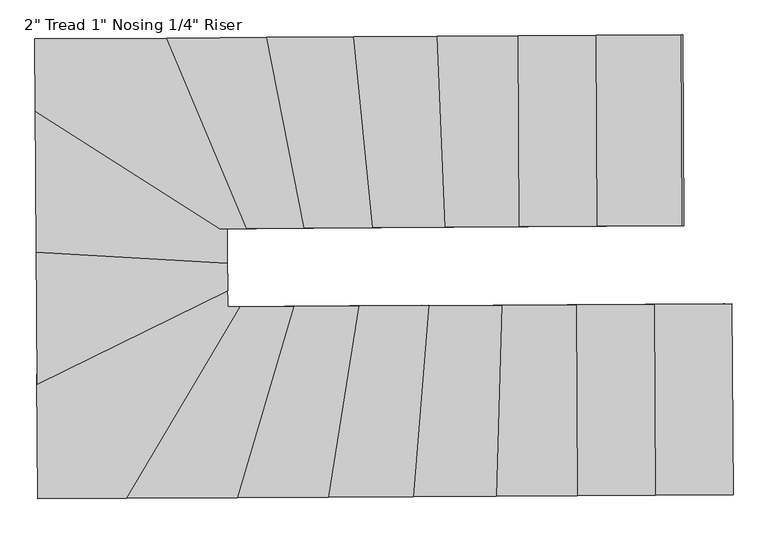
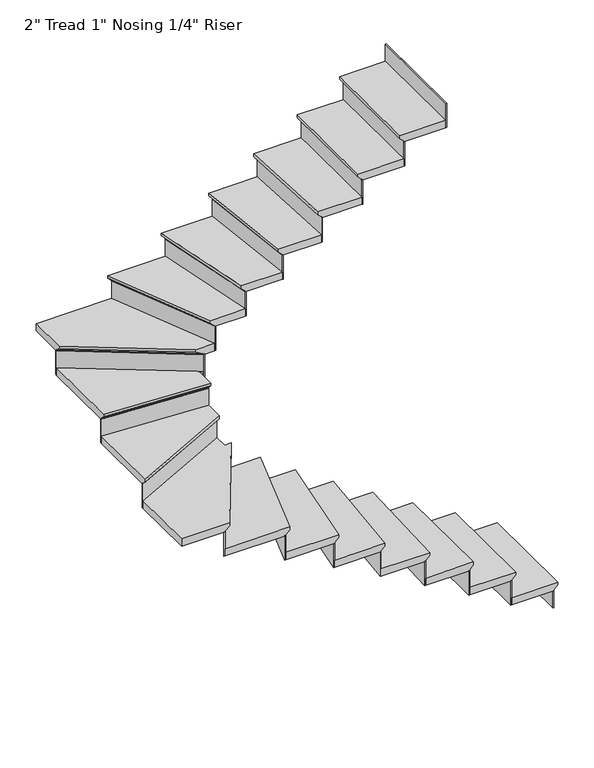
"""IFC4 building model written with IfcOpenShell, lengths in millimetres: stair flight geometry."""

from ifc_helpers import new_model, si_unit, origin, place, context, project, spatial, faceted_brep, source, transform, mapped, element, save


def stair_flight_f68b1b91(model_context):
    return source(origin(), model_context, "Body", "Brep", [
        faceted_brep([(-120.6930289, -3539.621908, 9751.4833333), (-120.6930289, -3539.621908, 9770.5333333), (-116.4891496, -4225.4090232, 9770.5333333), (-116.4891496, -4225.4090232, 9751.4833333), (-146.0925517, -3539.7776072, 9726.0833333), (-141.8886723, -4225.5647224, 9726.0833333), (-425.4873024, -3541.4902988, 9770.5333333), (-421.283423, -4227.277414, 9770.5333333), (-141.8886723, -4225.5647224, 9719.7333333), (-421.283423, -4227.277414, 9719.7333333), (-425.4873024, -3541.4902988, 9719.7333333), (-146.0925517, -3539.7776072, 9719.7333333)], [[[0, 1, 2, 3]], [[4, 0, 3, 5]], [[2, 1, 6, 7]], [[8, 9, 10, 11]], [[2, 7, 9, 8, 5, 3]], [[8, 11, 4, 5]], [[6, 1, 0, 4, 11, 10]], [[7, 6, 10, 9]]]),
        faceted_brep([(-146.0925517, -3539.7776072, 9719.7333333), (-146.0925517, -3539.7776072, 9601.2), (-152.4424324, -3539.816532, 9601.2), (-152.4424324, -3539.816532, 9719.7333333), (-141.8886723, -4225.5647224, 9719.7333333), (-148.238553, -4225.6036472, 9719.7333333), (-148.238553, -4225.6036472, 9601.2), (-141.8886723, -4225.5647224, 9601.2)], [[[0, 1, 2, 3]], [[4, 5, 6, 7]], [[1, 0, 4, 7]], [[2, 1, 7, 6]], [[3, 2, 6, 5]], [[0, 3, 5, 4]]]),
        faceted_brep([(-425.4873024, -3541.4902988, 9889.0666667), (-425.4873024, -3541.4902988, 9719.7333333), (-431.8371831, -3541.5292236, 9719.7333333), (-431.8371831, -3541.5292236, 9889.0666667), (-421.283423, -4227.277414, 9889.0666667), (-427.6333037, -4227.3163388, 9889.0666667), (-427.6333037, -4227.3163388, 9719.7333333), (-421.283423, -4227.277414, 9719.7333333)], [[[0, 1, 2, 3]], [[4, 5, 6, 7]], [[1, 0, 4, 7]], [[2, 1, 7, 6]], [[3, 2, 6, 5]], [[0, 3, 5, 4]]]),
        faceted_brep([(-395.8839002, -4227.1217148, 9939.8666667), (-400.0877796, -3541.3345996, 9939.8666667), (-704.882053, -3543.2029904, 9939.8666667), (-700.6781736, -4228.9901056, 9939.8666667), (-421.283423, -4227.277414, 9889.0666667), (-700.6781736, -4228.9901056, 9889.0666667), (-704.882053, -3543.2029904, 9889.0666667), (-425.4873024, -3541.4902988, 9889.0666667), (-421.283423, -4227.277414, 9895.4166667), (-395.8839002, -4227.1217148, 9920.8166667), (-425.4873024, -3541.4902988, 9895.4166667), (-400.0877796, -3541.3345996, 9920.8166667)], [[[0, 1, 2, 3]], [[4, 5, 6, 7]], [[0, 3, 5, 4, 8, 9]], [[4, 7, 10, 8]], [[2, 1, 11, 10, 7, 6]], [[3, 2, 6, 5]], [[11, 1, 0, 9]], [[10, 11, 9, 8]]]),
        faceted_brep([(-704.882053, -3543.2029904, 10058.4), (-704.882053, -3543.2029904, 9889.0666667), (-711.2319337, -3543.2419152, 9889.0666667), (-711.2319337, -3543.2419152, 10058.4), (-700.6781736, -4228.9901056, 10058.4), (-707.0280543, -4229.0290304, 10058.4), (-707.0280543, -4229.0290304, 9889.0666667), (-700.6781736, -4228.9901056, 9889.0666667)], [[[0, 1, 2, 3]], [[4, 5, 6, 7]], [[1, 0, 4, 7]], [[2, 1, 7, 6]], [[3, 2, 6, 5]], [[0, 3, 5, 4]]]),
        faceted_brep([(-675.2786508, -4228.8344064, 10109.2), (-679.4825302, -3543.0472912, 10109.2), (-971.9344004, -3544.840023, 10109.2), (-992.4483132, -4230.7786584, 10109.2), (-700.6781736, -4228.9901056, 10058.4), (-992.4483132, -4230.7786584, 10058.4), (-971.9344004, -3544.840023, 10058.4), (-704.882053, -3543.2029904, 10058.4), (-700.6781736, -4228.9901056, 10064.75), (-675.2786508, -4228.8344064, 10090.15), (-704.882053, -3543.2029904, 10064.75), (-679.4825302, -3543.0472912, 10090.15)], [[[0, 1, 2, 3]], [[4, 5, 6, 7]], [[0, 3, 5, 4, 8, 9]], [[4, 7, 10, 8]], [[2, 1, 11, 10, 7, 6]], [[3, 2, 6, 5]], [[11, 1, 0, 9]], [[10, 11, 9, 8]]]),
        faceted_brep([(-971.9344004, -3544.840023, 10227.7333333), (-971.9344004, -3544.840023, 10058.4), (-978.2884043, -3544.8789731, 10058.4), (-978.2884043, -3544.8789731, 10227.7333333), (-992.4483132, -4230.7786584, 10227.7333333), (-998.8023171, -4230.8176085, 10227.7333333), (-998.8023171, -4230.8176085, 10058.4), (-992.4483132, -4230.7786584, 10058.4)], [[[0, 1, 2, 3]], [[4, 5, 6, 7]], [[1, 0, 4, 7]], [[2, 1, 7, 6]], [[3, 2, 6, 5]], [[0, 3, 5, 4]]]),
        faceted_brep([(-967.0322975, -4230.6228581, 10278.5333333), (-946.5183848, -3544.6842227, 10278.5333333), (-1233.842238, -3546.4455197, 10278.5333333), (-1289.4900883, -4232.5995264, 10278.5333333), (-992.4483132, -4230.7786584, 10227.7333333), (-1289.4900883, -4232.5995264, 10227.7333333), (-1233.842238, -3546.4455197, 10227.7333333), (-971.9344004, -3544.840023, 10227.7333333), (-992.4483132, -4230.7786584, 10234.0833333), (-967.0322975, -4230.6228581, 10259.4833333), (-971.9344004, -3544.840023, 10234.0833333), (-946.5183848, -3544.6842227, 10259.4833333)], [[[0, 1, 2, 3]], [[4, 5, 6, 7]], [[0, 3, 5, 4, 8, 9]], [[4, 7, 10, 8]], [[2, 1, 11, 10, 7, 6]], [[3, 2, 6, 5]], [[11, 1, 0, 9]], [[10, 11, 9, 8]]]),
        faceted_brep([(-1233.842238, -3546.4455197, 10397.0666667), (-1233.842238, -3546.4455197, 10227.7333333), (-1240.2162558, -3546.4845925, 10227.7333333), (-1240.2162558, -3546.4845925, 10397.0666667), (-1289.4900883, -4232.5995264, 10397.0666667), (-1295.8641061, -4232.6385992, 10397.0666667), (-1295.8641061, -4232.6385992, 10227.7333333), (-1289.4900883, -4232.5995264, 10227.7333333)], [[[0, 1, 2, 3]], [[4, 5, 6, 7]], [[1, 0, 4, 7]], [[2, 1, 7, 6]], [[3, 2, 6, 5]], [[0, 3, 5, 4]]]),
        faceted_brep([(-1263.994017, -4232.4432353, 10447.8666667), (-1208.3461666, -3546.2892286, 10447.8666667), (-1486.5415383, -3547.994568, 10447.8666667), (-1596.081167, -4234.4789317, 10447.8666667), (-1289.4900883, -4232.5995264, 10397.0666667), (-1596.081167, -4234.4789317, 10397.0666667), (-1486.5415383, -3547.994568, 10397.0666667), (-1233.842238, -3546.4455197, 10397.0666667), (-1289.4900883, -4232.5995264, 10403.4166667), (-1263.994017, -4232.4432353, 10428.8166667), (-1233.842238, -3546.4455197, 10403.4166667), (-1208.3461666, -3546.2892286, 10428.8166667)], [[[0, 1, 2, 3]], [[4, 5, 6, 7]], [[0, 3, 5, 4, 8, 9]], [[4, 7, 10, 8]], [[2, 1, 11, 10, 7, 6]], [[3, 2, 6, 5]], [[11, 1, 0, 9]], [[10, 11, 9, 8]]]),
        faceted_brep([(-1486.5415383, -3547.994568, 10566.4), (-1486.5415383, -3547.994568, 10397.0666667), (-1492.9781659, -3548.0340246, 10397.0666667), (-1492.9781659, -3548.0340246, 10566.4), (-1596.081167, -4234.4789317, 10566.4), (-1602.5177946, -4234.5183882, 10566.4), (-1602.5177946, -4234.5183882, 10397.0666667), (-1596.081167, -4234.4789317, 10397.0666667)], [[[0, 1, 2, 3]], [[4, 5, 6, 7]], [[1, 0, 4, 7]], [[2, 1, 7, 6]], [[3, 2, 6, 5]], [[0, 3, 5, 4]]]),
        faceted_brep([(-1570.3346568, -4234.3211054, 10617.2), (-1460.7950281, -3547.8367418, 10617.2), (-1720.1488607, -3549.4265824, 10617.2), (-1922.8306159, -4236.4819079, 10617.2), (-1596.081167, -4234.4789317, 10566.4), (-1922.8306159, -4236.4819079, 10566.4), (-1720.1488607, -3549.4265824, 10566.4), (-1486.5415383, -3547.994568, 10566.4), (-1596.081167, -4234.4789317, 10572.75), (-1570.3346568, -4234.3211054, 10598.15), (-1486.5415383, -3547.994568, 10572.75), (-1460.7950281, -3547.8367418, 10598.15)], [[[0, 1, 2, 3]], [[4, 5, 6, 7]], [[0, 3, 5, 4, 8, 9]], [[4, 7, 10, 8]], [[2, 1, 11, 10, 7, 6]], [[3, 2, 6, 5]], [[11, 1, 0, 9]], [[10, 11, 9, 8]]]),
        faceted_brep([(-1720.1488607, -3549.4265824, 10735.7333333), (-1720.1488607, -3549.4265824, 10566.4), (-1726.781397, -3549.4672399, 10566.4), (-1726.781397, -3549.4672399, 10735.7333333), (-1922.8306159, -4236.4819079, 10735.7333333), (-1929.4631522, -4236.5225654, 10735.7333333), (-1929.4631522, -4236.5225654, 10566.4), (-1922.8306159, -4236.4819079, 10566.4)], [[[0, 1, 2, 3]], [[4, 5, 6, 7]], [[1, 0, 4, 7]], [[2, 1, 7, 6]], [[3, 2, 6, 5]], [[0, 3, 5, 4]]]),
        faceted_brep([(-1896.3004707, -4236.3192779, 10786.5333333), (-1693.6187155, -3549.2639524, 10786.5333333), (-1917.3665941, -3550.6355283, 10786.5333333), (-2324.8688668, -4238.9464049, 10786.5333333), (-1922.8306159, -4236.4819079, 10735.7333333), (-2324.8688668, -4238.9464049, 10735.7333333), (-1917.3665941, -3550.6355283, 10735.7333333), (-1720.1488607, -3549.4265824, 10735.7333333), (-1922.8306159, -4236.4819079, 10742.0833333), (-1896.3004707, -4236.3192779, 10767.4833333), (-1720.1488607, -3549.4265824, 10742.0833333), (-1693.6187155, -3549.2639524, 10767.4833333)], [[[0, 1, 2, 3]], [[4, 5, 6, 7]], [[0, 3, 5, 4, 8, 9]], [[4, 7, 10, 8]], [[2, 1, 11, 10, 7, 6]], [[3, 2, 6, 5]], [[11, 1, 0, 9]], [[10, 11, 9, 8]]]),
        faceted_brep([(-1917.3665941, -3550.6355283, 10905.0666667), (-1917.3665941, -3550.6355283, 10735.7333333), (-1924.7728783, -3550.6809289, 10735.7333333), (-1924.7728783, -3550.6809289, 10905.0666667), (-2324.8688668, -4238.9464049, 10905.0666667), (-2332.275151, -4238.9918055, 10905.0666667), (-2332.275151, -4238.9918055, 10735.7333333), (-2324.8688668, -4238.9464049, 10735.7333333)], [[[0, 1, 2, 3]], [[4, 5, 6, 7]], [[1, 0, 4, 7]], [[2, 1, 7, 6]], [[3, 2, 6, 5]], [[0, 3, 5, 4]]]),
        faceted_brep([(-2615.3480869, -3801.2875551, 10955.8666667), (-2612.6544213, -4240.7105322, 10955.8666667), (-2295.24373, -4238.7648026, 10955.8666667), (-1887.7414574, -3550.4539261, 10955.8666667), (-1931.0711854, -3550.7195376, 10955.8666667), (-1931.5966592, -3464.9979706, 10955.8666667), (-2612.6544213, -4240.7105322, 10905.0666667), (-2615.3480869, -3801.2875551, 10905.0666667), (-1931.5966592, -3464.9979706, 10905.0666667), (-1931.0711854, -3550.7195376, 10905.0666667), (-1917.3665941, -3550.6355283, 10905.0666667), (-2324.8688668, -4238.9464049, 10905.0666667), (-1917.3665941, -3550.6355283, 10911.4166667), (-2324.8688668, -4238.9464049, 10911.4166667), (-1887.7414574, -3550.4539261, 10936.8166667), (-2295.24373, -4238.7648026, 10936.8166667)], [[[0, 1, 2, 3, 4, 5]], [[6, 7, 8, 9, 10, 11]], [[1, 0, 7, 6]], [[11, 10, 12, 13]], [[5, 4, 9, 8]], [[0, 5, 8, 7]], [[14, 3, 2, 15]], [[12, 14, 15, 13]], [[4, 3, 14, 12, 10, 9]], [[2, 1, 6, 11, 13, 15]]]),
        faceted_brep([(-1931.5966592, -3464.9979706, 11074.4), (-1931.5966592, -3464.9979706, 10905.0666667), (-1931.6399076, -3457.9427742, 10905.0666667), (-1931.6399076, -3457.9427742, 11074.4), (-2615.3480869, -3801.2875551, 11074.4), (-2615.3913353, -3794.2323587, 11074.4), (-2615.3913353, -3794.2323587, 10905.0666667), (-2615.3480869, -3801.2875551, 10905.0666667)], [[[0, 1, 2, 3]], [[4, 5, 6, 7]], [[1, 0, 4, 7]], [[2, 1, 7, 6]], [[3, 2, 6, 5]], [[0, 3, 5, 4]]]),
        faceted_brep([(-2615.1750933, -3829.5083406, 11125.2), (-1931.4236656, -3493.2187561, 11125.2), (-1932.1828972, -3369.3638122, 11125.2), (-2618.2387587, -3329.7265819, 11125.2), (-2615.3480869, -3801.2875551, 11074.4), (-2618.2387587, -3329.7265819, 11074.4), (-1932.1828972, -3369.3638122, 11074.4), (-1931.5966592, -3464.9979706, 11074.4), (-2615.3480869, -3801.2875551, 11080.75), (-2615.1750933, -3829.5083406, 11106.15), (-1931.5966592, -3464.9979706, 11080.75), (-1931.4236656, -3493.2187561, 11106.15)], [[[0, 1, 2, 3]], [[4, 5, 6, 7]], [[0, 3, 5, 4, 8, 9]], [[4, 7, 10, 8]], [[2, 1, 11, 10, 7, 6]], [[3, 2, 6, 5]], [[11, 1, 0, 9]], [[10, 11, 9, 8]]]),
        faceted_brep([(-1932.1828972, -3369.3638122, 11243.7333333), (-1932.1828972, -3369.3638122, 11074.4), (-1932.2219015, -3363.0009693, 11074.4), (-1932.2219015, -3363.0009693, 11243.7333333), (-2618.2387587, -3329.7265819, 11243.7333333), (-2618.277763, -3323.363739, 11243.7333333), (-2618.277763, -3323.363739, 11074.4), (-2618.2387587, -3329.7265819, 11074.4)], [[[0, 1, 2, 3]], [[4, 5, 6, 7]], [[1, 0, 4, 7]], [[2, 1, 7, 6]], [[3, 2, 6, 5]], [[0, 3, 5, 4]]]),
        faceted_brep([(-2618.0827416, -3355.1779533, 11294.5333333), (-1932.0268801, -3394.8151835, 11294.5333333), (-1932.783877, -3271.3247869, 11294.5333333), (-1912.0496222, -3271.1976858, 11294.5333333), (-2621.364296, -2819.8515342, 11294.5333333), (-2618.2387587, -3329.7265819, 11243.7333333), (-2621.364296, -2819.8515342, 11243.7333333), (-1912.0496222, -3271.1976858, 11243.7333333), (-1932.783877, -3271.3247869, 11243.7333333), (-1932.1828972, -3369.3638122, 11243.7333333), (-2618.2387587, -3329.7265819, 11250.0833333), (-2618.0827416, -3355.1779533, 11275.4833333), (-1932.1828972, -3369.3638122, 11250.0833333), (-1932.0268801, -3394.8151835, 11275.4833333)], [[[0, 1, 2, 3, 4]], [[5, 6, 7, 8, 9]], [[0, 4, 6, 5, 10, 11]], [[5, 9, 12, 10]], [[2, 1, 13, 12, 9, 8]], [[3, 2, 8, 7]], [[4, 3, 7, 6]], [[13, 1, 0, 11]], [[12, 13, 11, 10]]]),
        faceted_brep([(-1912.0496222, -3271.1976858, 11413.0666667), (-1912.0496222, -3271.1976858, 11243.7333333), (-1900.3341194, -3271.1258697, 11243.7333333), (-1900.3341194, -3271.1258697, 11413.0666667), (-2621.364296, -2819.8515342, 11413.0666667), (-2621.4106144, -2812.2955182, 11413.0666667), (-2621.4106144, -2812.2955182, 11243.7333333), (-2621.364296, -2819.8515342, 11243.7333333)], [[[0, 1, 2, 3]], [[4, 5, 6, 7]], [[1, 0, 4, 7]], [[2, 1, 7, 6]], [[3, 2, 6, 5]], [[0, 3, 5, 4]]]),
        faceted_brep([(-2121.4312205, -2586.6683113, 11463.8666667), (-2622.7748716, -2589.7415511, 11463.8666667), (-2621.1790223, -2850.0755978, 11463.8666667), (-1958.9116334, -3271.4849502, 11463.8666667), (-1835.3232791, -3270.7273529, 11463.8666667), (-2622.7748716, -2589.7415511, 11413.0666667), (-2121.4312205, -2586.6683113, 11413.0666667), (-1835.3232791, -3270.7273529, 11413.0666667), (-1912.0496222, -3271.1976858, 11413.0666667), (-2621.364296, -2819.8515342, 11413.0666667), (-2621.364296, -2819.8515342, 11419.4166667), (-2621.1790223, -2850.0755978, 11444.8166667), (-1912.0496222, -3271.1976858, 11419.4166667), (-1958.9116334, -3271.4849502, 11444.8166667)], [[[0, 1, 2, 3, 4]], [[5, 6, 7, 8, 9]], [[1, 0, 6, 5]], [[2, 1, 5, 9, 10, 11]], [[9, 8, 12, 10]], [[0, 4, 7, 6]], [[13, 3, 2, 11]], [[12, 13, 11, 10]], [[4, 3, 13, 12, 8, 7]]]),
        faceted_brep([(-1835.3232791, -3270.7273529, 11582.4), (-1835.3232791, -3270.7273529, 11413.0666667), (-1828.4578405, -3270.6852677, 11413.0666667), (-1828.4578405, -3270.6852677, 11582.4), (-2121.4312205, -2586.6683113, 11582.4), (-2114.5657819, -2586.6262261, 11582.4), (-2114.5657819, -2586.6262261, 11413.0666667), (-2121.4312205, -2586.6683113, 11413.0666667)], [[[0, 1, 2, 3]], [[4, 5, 6, 7]], [[1, 0, 4, 7]], [[2, 1, 7, 6]], [[3, 2, 6, 5]], [[0, 3, 5, 4]]]),
        faceted_brep([(-2148.8929752, -2586.8366521, 11633.2), (-1862.7850338, -3270.8956936, 11633.2), (-1630.6514822, -3269.4727134, 11633.2), (-1765.0751589, -2584.4838464, 11633.2), (-2121.4312205, -2586.6683113, 11582.4), (-1765.0751589, -2584.4838464, 11582.4), (-1630.6514822, -3269.4727134, 11582.4), (-1835.3232791, -3270.7273529, 11582.4), (-2121.4312205, -2586.6683113, 11588.75), (-2148.8929752, -2586.8366521, 11614.15), (-1835.3232791, -3270.7273529, 11588.75), (-1862.7850338, -3270.8956936, 11614.15)], [[[0, 1, 2, 3]], [[4, 5, 6, 7]], [[0, 3, 5, 4, 8, 9]], [[4, 7, 10, 8]], [[2, 1, 11, 10, 7, 6]], [[3, 2, 6, 5]], [[11, 1, 0, 9]], [[10, 11, 9, 8]]]),
        faceted_brep([(-1630.6514822, -3269.4727134, 11751.7333333), (-1630.6514822, -3269.4727134, 11582.4), (-1624.1881401, -3269.4330931, 11582.4), (-1624.1881401, -3269.4330931, 11751.7333333), (-1765.0751589, -2584.4838464, 11751.7333333), (-1758.6118168, -2584.4442261, 11751.7333333), (-1758.6118168, -2584.4442261, 11582.4), (-1765.0751589, -2584.4838464, 11582.4)], [[[0, 1, 2, 3]], [[4, 5, 6, 7]], [[1, 0, 4, 7]], [[2, 1, 7, 6]], [[3, 2, 6, 5]], [[0, 3, 5, 4]]]),
        faceted_brep([(-1790.9285273, -2584.6423277, 11802.5333333), (-1656.5048506, -3269.6311948, 11802.5333333), (-1385.319119, -3267.9688245, 11802.5333333), (-1452.3132293, -2582.5666138, 11802.5333333), (-1765.0751589, -2584.4838464, 11751.7333333), (-1452.3132293, -2582.5666138, 11751.7333333), (-1385.319119, -3267.9688245, 11751.7333333), (-1630.6514822, -3269.4727134, 11751.7333333), (-1765.0751589, -2584.4838464, 11758.0833333), (-1790.9285273, -2584.6423277, 11783.4833333), (-1630.6514822, -3269.4727134, 11758.0833333), (-1656.5048506, -3269.6311948, 11783.4833333)], [[[0, 1, 2, 3]], [[4, 5, 6, 7]], [[0, 3, 5, 4, 8, 9]], [[4, 7, 10, 8]], [[2, 1, 11, 10, 7, 6]], [[3, 2, 6, 5]], [[11, 1, 0, 9]], [[10, 11, 9, 8]]]),
        faceted_brep([(-1385.319119, -3267.9688245, 11921.0666667), (-1385.319119, -3267.9688245, 11751.7333333), (-1378.942678, -3267.9297369, 11751.7333333), (-1378.942678, -3267.9297369, 11921.0666667), (-1452.3132293, -2582.5666138, 11921.0666667), (-1445.9367882, -2582.5275262, 11921.0666667), (-1445.9367882, -2582.5275262, 11751.7333333), (-1452.3132293, -2582.5666138, 11751.7333333)], [[[0, 1, 2, 3]], [[4, 5, 6, 7]], [[1, 0, 4, 7]], [[2, 1, 7, 6]], [[3, 2, 6, 5]], [[0, 3, 5, 4]]]),
        faceted_brep([(-1477.8189934, -2582.7229643, 11971.8666667), (-1410.8248832, -3268.125175, 11971.8666667), (-1125.1141805, -3266.3737666, 11971.8666667), (-1153.9085026, -2580.7373909, 11971.8666667), (-1452.3132293, -2582.5666138, 11921.0666667), (-1153.9085026, -2580.7373909, 11921.0666667), (-1125.1141805, -3266.3737666, 11921.0666667), (-1385.319119, -3267.9688245, 11921.0666667), (-1452.3132293, -2582.5666138, 11927.4166667), (-1477.8189934, -2582.7229643, 11952.8166667), (-1385.319119, -3267.9688245, 11927.4166667), (-1410.8248832, -3268.125175, 11952.8166667)], [[[0, 1, 2, 3]], [[4, 5, 6, 7]], [[0, 3, 5, 4, 8, 9]], [[4, 7, 10, 8]], [[2, 1, 11, 10, 7, 6]], [[3, 2, 6, 5]], [[11, 1, 0, 9]], [[10, 11, 9, 8]]]),
        faceted_brep([(-1125.1141805, -3266.3737666, 12090.4), (-1125.1141805, -3266.3737666, 11921.0666667), (-1118.7602189, -3266.3348167, 11921.0666667), (-1118.7602189, -3266.3348167, 12090.4), (-1153.9085026, -2580.7373909, 12090.4), (-1147.554541, -2580.6984411, 12090.4), (-1147.554541, -2580.6984411, 11921.0666667), (-1153.9085026, -2580.7373909, 11921.0666667)], [[[0, 1, 2, 3]], [[4, 5, 6, 7]], [[1, 0, 4, 7]], [[2, 1, 7, 6]], [[3, 2, 6, 5]], [[0, 3, 5, 4]]]),
        faceted_brep([(-1179.3243487, -2580.8931902, 12141.2), (-1150.5300267, -3266.5295659, 12141.2), (-858.0309746, -3264.7365448, 12141.2), (-862.2348539, -2578.9494296, 12141.2), (-1153.9085026, -2580.7373909, 12090.4), (-862.2348539, -2578.9494296, 12090.4), (-858.0309746, -3264.7365448, 12090.4), (-1125.1141805, -3266.3737666, 12090.4), (-1153.9085026, -2580.7373909, 12096.75), (-1179.3243487, -2580.8931902, 12122.15), (-1125.1141805, -3266.3737666, 12096.75), (-1150.5300267, -3266.5295659, 12122.15)], [[[0, 1, 2, 3]], [[4, 5, 6, 7]], [[0, 3, 5, 4, 8, 9]], [[4, 7, 10, 8]], [[2, 1, 11, 10, 7, 6]], [[3, 2, 6, 5]], [[11, 1, 0, 9]], [[10, 11, 9, 8]]]),
        faceted_brep([(-858.0309746, -3264.7365448, 12259.7333333), (-858.0309746, -3264.7365448, 12090.4), (-851.6810939, -3264.69762, 12090.4), (-851.6810939, -3264.69762, 12259.7333333), (-862.2348539, -2578.9494296, 12259.7333333), (-855.8849733, -2578.9105048, 12259.7333333), (-855.8849733, -2578.9105048, 12090.4), (-862.2348539, -2578.9494296, 12090.4)], [[[0, 1, 2, 3]], [[4, 5, 6, 7]], [[1, 0, 4, 7]], [[2, 1, 7, 6]], [[3, 2, 6, 5]], [[0, 3, 5, 4]]]),
        faceted_brep([(-887.6343767, -2579.1051288, 12310.5333333), (-883.4304974, -3264.8922441, 12310.5333333), (-578.6362239, -3263.0238532, 12310.5333333), (-582.8401033, -2577.236738, 12310.5333333), (-862.2348539, -2578.9494296, 12259.7333333), (-582.8401033, -2577.236738, 12259.7333333), (-578.6362239, -3263.0238532, 12259.7333333), (-858.0309746, -3264.7365448, 12259.7333333), (-862.2348539, -2578.9494296, 12266.0833333), (-887.6343767, -2579.1051288, 12291.4833333), (-858.0309746, -3264.7365448, 12266.0833333), (-883.4304974, -3264.8922441, 12291.4833333)], [[[0, 1, 2, 3]], [[4, 5, 6, 7]], [[0, 3, 5, 4, 8, 9]], [[4, 7, 10, 8]], [[2, 1, 11, 10, 7, 6]], [[3, 2, 6, 5]], [[11, 1, 0, 9]], [[10, 11, 9, 8]]]),
        faceted_brep([(-578.6362239, -3263.0238532, 12429.0666667), (-578.6362239, -3263.0238532, 12259.7333333), (-572.2863432, -3262.9849284, 12259.7333333), (-572.2863432, -3262.9849284, 12429.0666667), (-582.8401033, -2577.236738, 12429.0666667), (-576.4902226, -2577.1978132, 12429.0666667), (-576.4902226, -2577.1978132, 12259.7333333), (-582.8401033, -2577.236738, 12259.7333333)], [[[0, 1, 2, 3]], [[4, 5, 6, 7]], [[1, 0, 4, 7]], [[2, 1, 7, 6]], [[3, 2, 6, 5]], [[0, 3, 5, 4]]]),
        faceted_brep([(-299.2414733, -3261.3111616, 12598.4), (-299.2414733, -3261.3111616, 12429.0666667), (-292.8915926, -3261.2722368, 12429.0666667), (-292.8915926, -3261.2722368, 12598.4), (-303.4453527, -2575.5240464, 12598.4), (-297.095472, -2575.4851216, 12598.4), (-297.095472, -2575.4851216, 12429.0666667), (-303.4453527, -2575.5240464, 12429.0666667)], [[[0, 1, 2, 3]], [[4, 5, 6, 7]], [[1, 0, 4, 7]], [[2, 1, 7, 6]], [[3, 2, 6, 5]], [[0, 3, 5, 4]]]),
        faceted_brep([(-608.2396261, -2577.3924372, 12479.8666667), (-604.0357467, -3263.1795525, 12479.8666667), (-299.2414733, -3261.3111616, 12479.8666667), (-303.4453527, -2575.5240464, 12479.8666667), (-582.8401033, -2577.236738, 12429.0666667), (-303.4453527, -2575.5240464, 12429.0666667), (-299.2414733, -3261.3111616, 12429.0666667), (-578.6362239, -3263.0238532, 12429.0666667), (-582.8401033, -2577.236738, 12435.4166667), (-608.2396261, -2577.3924372, 12460.8166667), (-578.6362239, -3263.0238532, 12435.4166667), (-604.0357467, -3263.1795525, 12460.8166667)], [[[0, 1, 2, 3]], [[4, 5, 6, 7]], [[0, 3, 5, 4, 8, 9]], [[4, 7, 10, 8]], [[2, 1, 11, 10, 7, 6]], [[3, 2, 6, 5]], [[11, 1, 0, 9]], [[10, 11, 9, 8]]]),
    ])


if __name__ == "__main__":
    model = new_model("IFC4")
    model_context = context("Model", 3, world=origin())
    ifc_project = project(units=[si_unit("LENGTHUNIT", "METRE", prefix="MILLI")], contexts=[model_context])
    site = spatial("IfcSite", under=ifc_project)
    building = spatial("IfcBuilding", under=site)
    placement = place(None, origin())
    stair_flight_shape = stair_flight_f68b1b91(model_context)
    element("IfcStairFlight", 1, ObjectType="2\" Tread 1\" Nosing 1/4\" Riser", at=placement, inside=building, context=model_context, shape_type="MappedRepresentation", body=[
        mapped(stair_flight_shape, transform((0.0, 0.0, 0.0), x_axis=(1.0, 0.0, 0.0), y_axis=(0.0, 1.0, 0.0), z_axis=(0.0, 0.0, 1.0))),
    ])
    save(model, "model.ifc")

# Revit data of these elements
# Element 1 (IfcStairFlight, "2\" Tread 1\" Nosing 1/4\" Riser")
#   Materials on its faces: "Door - Frame"
# Materials
#   "Door - Frame": colour RGB 118 70 51, transparency 0, Cost = 0
